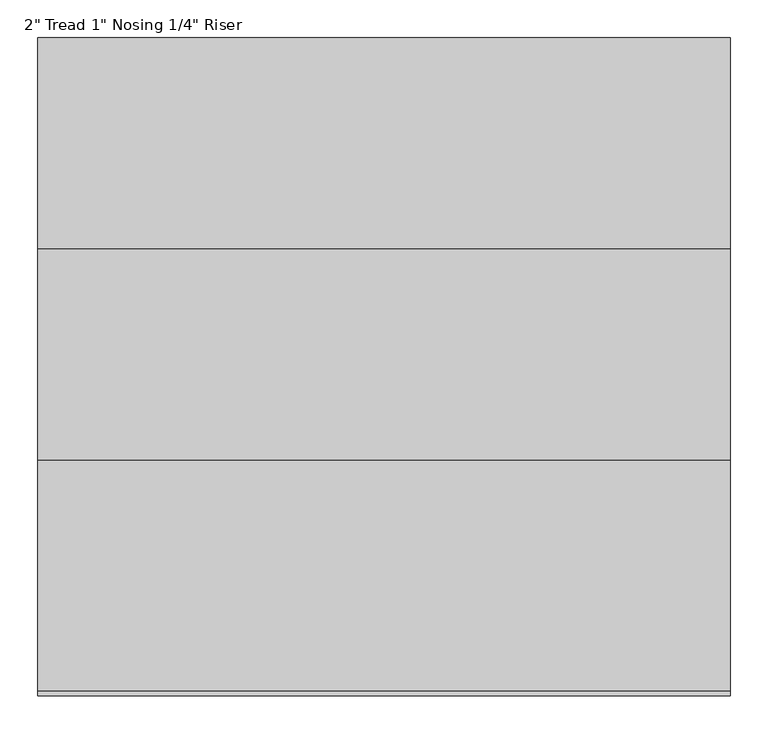
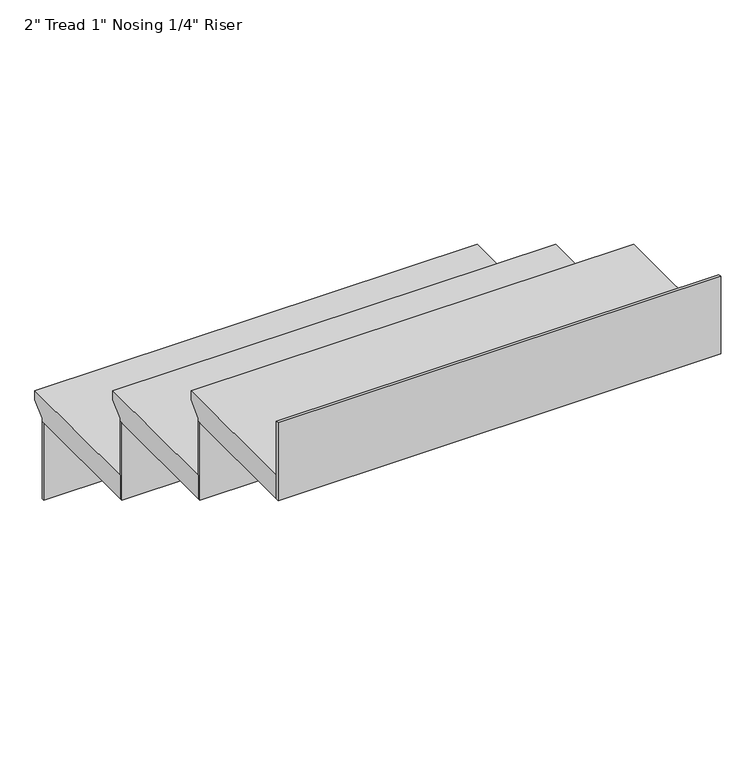
"""IFC4 building model written with IfcOpenShell, lengths in millimetres: stair flight geometry."""

from ifc_helpers import new_model, si_unit, frame, origin, place, context, project, spatial, polyline, outline, extrude, source, transform, mapped, element, save


def stair_flight_e6b75d85(model_context):
    return source(origin(), model_context, "Body", "SweptSolid", [
        extrude(outline(polyline([(-19826.9851539, 30822.6172466), (-19522.1851539, 30822.6172466), (-19522.1851539, 30803.5672466), (-19547.5851539, 30778.1672466), (-19547.5851539, 30771.8172466), (-19826.9851539, 30771.8172466), (-19826.9851539, 30822.6172466)])), frame((-2296.6415084, 0.0, 0.0), z_axis=(1.0, 0.0, 0.0), x_axis=(0.0, 1.0, 0.0)), (0.0, 0.0, 1.0), 914.4),
        extrude(outline(polyline([(-2296.6415084, -19553.9351539), (-2296.6415084, -19547.5851539), (-1382.2415084, -19547.5851539), (-1382.2415084, -19553.9351539), (-2296.6415084, -19553.9351539)])), frame((0.0, 0.0, 30602.4839133), z_axis=(0.0, 0.0, 1.0), x_axis=(1.0, 0.0, 0.0)), (0.0, 0.0, 1.0), 169.3333333),
        extrude(outline(polyline([(-2296.6415084, -19833.3351539), (-2296.6415084, -19826.9851539), (-1382.2415084, -19826.9851539), (-1382.2415084, -19833.3351539), (-2296.6415084, -19833.3351539)])), frame((0.0, 0.0, 30771.8172466), z_axis=(0.0, 0.0, 1.0), x_axis=(1.0, 0.0, 0.0)), (0.0, 0.0, 1.0), 169.3333333),
        extrude(outline(polyline([(-20106.3851539, 30991.9505799), (-19801.5851539, 30991.9505799), (-19801.5851539, 30972.9005799), (-19826.9851539, 30947.5005799), (-19826.9851539, 30941.1505799), (-20106.3851539, 30941.1505799), (-20106.3851539, 30991.9505799)])), frame((-2296.6415084, 0.0, 0.0), z_axis=(1.0, 0.0, 0.0), x_axis=(0.0, 1.0, 0.0)), (0.0, 0.0, 1.0), 914.4),
        extrude(outline(polyline([(-2296.6415084, -20112.7351539), (-2296.6415084, -20106.3851539), (-1382.2415084, -20106.3851539), (-1382.2415084, -20112.7351539), (-2296.6415084, -20112.7351539)])), frame((0.0, 0.0, 30941.1505799), z_axis=(0.0, 0.0, 1.0), x_axis=(1.0, 0.0, 0.0)), (0.0, 0.0, 1.0), 169.3333333),
        extrude(outline(polyline([(-2296.6415084, -20392.1351539), (-2296.6415084, -20385.7851539), (-1382.2415084, -20385.7851539), (-1382.2415084, -20392.1351539), (-2296.6415084, -20392.1351539)])), frame((0.0, 0.0, 31110.4839133), z_axis=(0.0, 0.0, 1.0), x_axis=(1.0, 0.0, 0.0)), (0.0, 0.0, 1.0), 169.3333333),
        extrude(outline(polyline([(-20385.7851539, 31161.2839133), (-20080.9851539, 31161.2839133), (-20080.9851539, 31142.2339133), (-20106.3851539, 31116.8339133), (-20106.3851539, 31110.4839133), (-20385.7851539, 31110.4839133), (-20385.7851539, 31161.2839133)])), frame((-2296.6415084, 0.0, 0.0), z_axis=(1.0, 0.0, 0.0), x_axis=(0.0, 1.0, 0.0)), (0.0, 0.0, 1.0), 914.4),
    ])


if __name__ == "__main__":
    model = new_model("IFC4")
    model_context = context("Model", 3, world=origin())
    ifc_project = project(units=[si_unit("LENGTHUNIT", "METRE", prefix="MILLI")], contexts=[model_context])
    site = spatial("IfcSite", under=ifc_project)
    building = spatial("IfcBuilding", under=site)
    placement = place(None, origin())
    stair_flight_shape = stair_flight_e6b75d85(model_context)
    element("IfcStairFlight", 1, ObjectType="2\" Tread 1\" Nosing 1/4\" Riser", at=placement, inside=building, context=model_context, shape_type="MappedRepresentation", body=[
        mapped(stair_flight_shape, transform((0.0, 0.0, 0.0), x_axis=(1.0, 0.0, 0.0), y_axis=(0.0, 1.0, 0.0), z_axis=(0.0, 0.0, 1.0))),
    ])
    save(model, "model.ifc")
